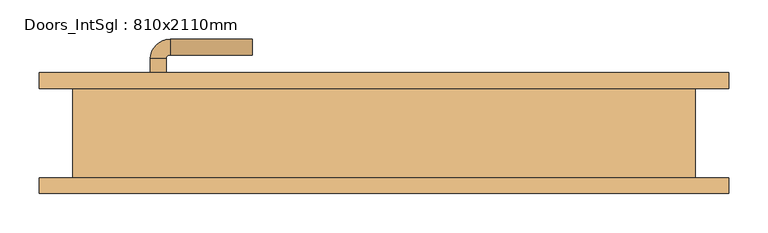
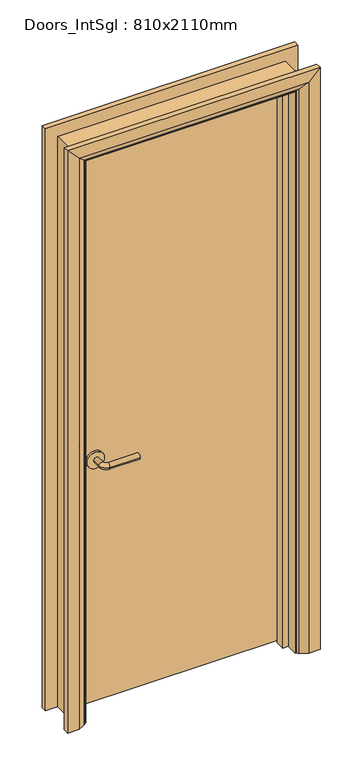
"""IFC4 building model written with IfcOpenShell, lengths in millimetres: door geometry, Doors_IntSgl : 810x2110mm."""

from ifc_helpers import new_model, si_unit, point, frame, frame_2d, origin, place, context, project, spatial, polyline, circle_curve, ellipse_curve, trimmed, segment, composite_curve, outline, extrude, faceted_brep, source, transform, mapped, element, save
from ifc_brep_helpers import plane_surface, cylinder_surface, revolved_surface, advanced_brep


def doors_intsgl_810x2110mm_5b69c0fd(model_context):
    return source(origin(), model_context, "Body", "SolidModel", [
        advanced_brep(
        [(-298.0, 11.15, 900.0), (-278.0, 11.15, 900.0), (-278.0, -18.85, 900.0), (-298.0, -18.85, 900.0), (-273.0, -23.85, 900.0), (-273.0, -43.85, 900.0), (-168.0, -43.85, 900.0), (-168.0, -23.85, 900.0)],
        [
            (0, 1, circle_curve(frame((-288.0, 11.15, 900.0), z_axis=(0.0, 1.0, 0.0), x_axis=(1.0, 0.0, 0.0)), 10.0)),
            (1, 0, circle_curve(frame((-288.0, 11.15, 900.0), z_axis=(0.0, 1.0, 0.0), x_axis=(1.0, 0.0, 0.0)), 10.0)),
            (1, 2),
            (2, 3, circle_curve(frame((-288.0, -18.85, 900.0), z_axis=(0.0, 1.0, 0.0), x_axis=(1.0, 0.0, 0.0)), 10.0)),
            (3, 0),
            (3, 2, circle_curve(frame((-288.0, -18.85, 900.0), z_axis=(0.0, 1.0, 0.0), x_axis=(1.0, 0.0, 0.0)), 10.0)),
            (4, 5, circle_curve(frame((-273.0, -33.85, 900.0), z_axis=(-1.0, 0.0, 0.0), x_axis=(0.0, 1.0, 0.0)), 10.0)),
            (5, 3, circle_curve(frame((-273.0, -18.85, 900.0), z_axis=(0.0, 0.0, -1.0), x_axis=(-1.0, 0.0, 0.0)), 25.0)),
            (2, 4, circle_curve(frame((-273.0, -18.85, 900.0), z_axis=(0.0, 0.0, 1.0), x_axis=(-1.0, 0.0, 0.0)), 5.0)),
            (5, 4, circle_curve(frame((-273.0, -33.85, 900.0), z_axis=(-1.0, 0.0, 0.0), x_axis=(0.0, 1.0, 0.0)), 10.0)),
            (6, 7, circle_curve(frame((-168.0, -33.85, 900.0), z_axis=(1.0, 0.0, 0.0), x_axis=(0.0, 1.0, 0.0)), 10.0)),
            (7, 6, circle_curve(frame((-168.0, -33.85, 900.0), z_axis=(1.0, 0.0, 0.0), x_axis=(0.0, 1.0, 0.0)), 10.0)),
            (4, 7),
            (6, 5),
        ],
        [
            plane_surface(frame((-288.0, 11.15, 900.0), z_axis=(0.0, 1.0, 0.0), x_axis=(0.0, 0.0, 1.0))),
            cylinder_surface(frame((-288.0, 11.15, 900.0), z_axis=(0.0, 1.0, 0.0), x_axis=(1.0, 0.0, 0.0)), 10.0),
            revolved_surface(trimmed(ellipse_curve(frame((-288.0, -18.85, 900.0), z_axis=(0.0, -1.0, 0.0), x_axis=(1.0, 0.0, 0.0)), 10.0, 10.0), [point((-298.0, -18.85, 900.0))], [point((-278.0, -18.85, 900.0))], True, "CARTESIAN"), (-273.0, -18.85, 900.0), (0.0, 0.0, -1.0)),
            revolved_surface(trimmed(ellipse_curve(frame((-288.0, -18.85, 900.0), z_axis=(0.0, -1.0, 0.0), x_axis=(1.0, 0.0, 0.0)), 10.0, 10.0), [point((-278.0, -18.85, 900.0))], [point((-298.0, -18.85, 900.0))], True, "CARTESIAN"), (-273.0, -18.85, 900.0), (0.0, 0.0, -1.0)),
            plane_surface(frame((-168.0, -33.85, 900.0), z_axis=(1.0, 0.0, 0.0), x_axis=(0.0, 0.0, 1.0))),
            cylinder_surface(frame((-273.0, -33.85, 900.0), z_axis=(-1.0, 0.0, 0.0), x_axis=(0.0, 1.0, 0.0)), 10.0),
        ],
        [
            (0, [[1, 2]]),
            (1, [[3, 4, 5, -2]]),
            (1, [[-5, 6, -3, -1]]),
            (2, [[7, 8, -4, 9]]),
            (3, [[10, -9, -6, -8]]),
            (4, [[11, 12]]),
            (5, [[13, -11, 14, -7]]),
            (5, [[-14, -12, -13, -10]]),
        ],
    ),
        extrude(outline(composite_curve([segment(trimmed(circle_curve(frame_2d((900.0, -290.5)), 30.0), [point((900.0, -320.5))], [point((900.0, -260.5))], False, "CARTESIAN"), True, "CONTINUOUS"), segment(trimmed(circle_curve(frame_2d((900.0, -290.5)), 30.0), [point((900.0, -260.5))], [point((900.0, -320.5))], False, "CARTESIAN"), True, "CONTINUOUS")], self_intersect=False)), frame((0.0, 11.15, 0.0), z_axis=(0.0, 1.0, 0.0), x_axis=(0.0, 0.0, 1.0)), (0.0, 0.0, 1.0), 8.0),
        advanced_brep(
        [(-298.0, 65.15, 900.0), (-278.0, 65.15, 900.0), (-298.0, 95.15, 900.0), (-278.0, 95.15, 900.0), (-273.0, 100.15, 900.0), (-273.0, 120.15, 900.0), (-168.0, 120.15, 900.0), (-168.0, 100.15, 900.0)],
        [
            (0, 1, circle_curve(frame((-288.0, 65.15, 900.0), z_axis=(0.0, -1.0, 0.0), x_axis=(1.0, 0.0, 0.0)), 10.0)),
            (1, 0, circle_curve(frame((-288.0, 65.15, 900.0), z_axis=(0.0, -1.0, 0.0), x_axis=(1.0, 0.0, 0.0)), 10.0)),
            (0, 2),
            (2, 3, circle_curve(frame((-288.0, 95.15, 900.0), z_axis=(0.0, -1.0, 0.0), x_axis=(1.0, 0.0, 0.0)), 10.0)),
            (3, 1),
            (3, 2, circle_curve(frame((-288.0, 95.15, 900.0), z_axis=(0.0, -1.0, 0.0), x_axis=(1.0, 0.0, 0.0)), 10.0)),
            (4, 3, circle_curve(frame((-273.0, 95.15, 900.0), z_axis=(0.0, 0.0, 1.0), x_axis=(-1.0, 0.0, 0.0)), 5.0)),
            (2, 5, circle_curve(frame((-273.0, 95.15, 900.0), z_axis=(0.0, 0.0, -1.0), x_axis=(-1.0, 0.0, 0.0)), 25.0)),
            (5, 4, circle_curve(frame((-273.0, 110.15, 900.0), z_axis=(-1.0, 0.0, 0.0), x_axis=(0.0, -1.0, 0.0)), 10.0)),
            (4, 5, circle_curve(frame((-273.0, 110.15, 900.0), z_axis=(-1.0, 0.0, 0.0), x_axis=(0.0, -1.0, 0.0)), 10.0)),
            (6, 7, circle_curve(frame((-168.0, 110.15, 900.0), z_axis=(1.0, 0.0, 0.0), x_axis=(0.0, -1.0, 0.0)), 10.0)),
            (7, 6, circle_curve(frame((-168.0, 110.15, 900.0), z_axis=(1.0, 0.0, 0.0), x_axis=(0.0, -1.0, 0.0)), 10.0)),
            (5, 6),
            (7, 4),
        ],
        [
            plane_surface(frame((-288.0, 65.15, 900.0), z_axis=(0.0, -1.0, 0.0), x_axis=(0.0, 0.0, 1.0))),
            cylinder_surface(frame((-288.0, 65.15, 900.0), z_axis=(0.0, -1.0, 0.0), x_axis=(1.0, 0.0, 0.0)), 10.0),
            revolved_surface(trimmed(ellipse_curve(frame((-288.0, 95.15, 900.0), z_axis=(0.0, -1.0, 0.0), x_axis=(1.0, 0.0, 0.0)), 10.0, 10.0), [point((-298.0, 95.15, 900.0))], [point((-278.0, 95.15, 900.0))], True, "CARTESIAN"), (-273.0, 95.15, 900.0), (0.0, 0.0, -1.0)),
            revolved_surface(trimmed(ellipse_curve(frame((-288.0, 95.15, 900.0), z_axis=(0.0, -1.0, 0.0), x_axis=(1.0, 0.0, 0.0)), 10.0, 10.0), [point((-278.0, 95.15, 900.0))], [point((-298.0, 95.15, 900.0))], True, "CARTESIAN"), (-273.0, 95.15, 900.0), (0.0, 0.0, -1.0)),
            plane_surface(frame((-168.0, 110.15, 900.0), z_axis=(1.0, 0.0, 0.0), x_axis=(0.0, 0.0, 1.0))),
            cylinder_surface(frame((-273.0, 110.15, 900.0), z_axis=(-1.0, 0.0, 0.0), x_axis=(0.0, -1.0, 0.0)), 10.0),
        ],
        [
            (0, [[1, 2]]),
            (1, [[-1, 3, 4, 5]]),
            (1, [[-2, -5, 6, -3]]),
            (2, [[7, -4, 8, 9]]),
            (3, [[-8, -6, -7, 10]]),
            (4, [[11, 12]]),
            (5, [[-9, 13, -12, 14]]),
            (5, [[-10, -14, -11, -13]]),
        ],
    ),
        extrude(outline(composite_curve([segment(trimmed(circle_curve(frame_2d((900.0, -290.5)), 30.0), [point((900.0, -320.5))], [point((900.0, -260.5))], False, "CARTESIAN"), True, "CONTINUOUS"), segment(trimmed(circle_curve(frame_2d((900.0, -290.5)), 30.0), [point((900.0, -260.5))], [point((900.0, -320.5))], False, "CARTESIAN"), True, "CONTINUOUS")], self_intersect=False)), frame((0.0, 57.15, 0.0), z_axis=(0.0, 1.0, 0.0), x_axis=(0.0, 0.0, 1.0)), (0.0, 0.0, 1.0), 8.0),
        extrude(outline(polyline([(363.0, 19.15), (-363.0, 19.15), (-363.0, 57.15), (363.0, 57.15), (363.0, 19.15)])), frame((0.0, 0.0, 8.0), z_axis=(0.0, 0.0, 1.0), x_axis=(1.0, 0.0, 0.0)), (0.0, 0.0, 1.0), 2060.0),
        advanced_brep(
        [(440.0, 77.15, 0.0), (440.0, 57.15, 0.0), (370.0, 57.15, 0.0), (374.0, 63.15, 0.0), (400.0, 77.15, 0.0), (440.0, 77.15, 2145.0), (440.0, 57.15, 2145.0), (-440.0, 57.15, 2145.0), (-440.0, 57.15, 0.0), (-370.0, 57.15, 0.0), (-370.0, 57.15, 2075.0), (370.0, 57.15, 2075.0), (374.0, 63.15, 2079.0), (400.0, 77.15, 2105.0), (-400.0, 77.15, 2105.0), (-400.0, 77.15, 0.0), (-440.0, 77.15, 0.0), (-440.0, 77.15, 2145.0), (-374.0, 63.15, 2079.0), (-374.0, 63.15, 0.0)],
        [
            (0, 1),
            (1, 2),
            (2, 3, circle_curve(frame((378.0, 56.15, 0.0), z_axis=(0.0, 0.0, -1.0), x_axis=(1.0, 0.0, 0.0)), 8.0622577)),
            (3, 4),
            (4, 0),
            (0, 5),
            (5, 6),
            (6, 1),
            (6, 7),
            (7, 8),
            (8, 9),
            (9, 10),
            (10, 11),
            (11, 2),
            (11, 12, ellipse_curve(frame((378.0, 56.15, 2083.0), z_axis=(0.7071067811865475, 0.0, -0.7071067811865475), x_axis=(-0.7071067811865474, 0.0, -0.7071067811865476)), 11.4017543, 8.0622577)),
            (12, 3),
            (12, 13),
            (13, 4),
            (13, 14),
            (14, 15),
            (15, 16),
            (16, 17),
            (17, 5),
            (17, 7),
            (10, 18, ellipse_curve(frame((-378.0, 56.15, 2083.0), z_axis=(0.7071067811865475, 0.0, 0.7071067811865475), x_axis=(0.7071067811865476, 0.0, -0.7071067811865474)), 11.4017543, 8.0622577)),
            (18, 12),
            (18, 14),
            (15, 19),
            (19, 9, circle_curve(frame((-378.0, 56.15, 0.0), z_axis=(0.0, 0.0, -1.0), x_axis=(-1.0, 0.0, 0.0)), 8.0622577)),
            (8, 16),
            (19, 18),
        ],
        [
            plane_surface(frame((370.0, 57.15, 0.0), z_axis=(0.0, 0.0, -1.0), x_axis=(0.0, -1.0, 0.0))),
            plane_surface(frame((440.0, 77.15, 0.0), z_axis=(1.0, 0.0, 0.0), x_axis=(0.0, 0.0, 1.0))),
            plane_surface(frame((440.0, 57.15, 0.0), z_axis=(0.0, -1.0, 0.0), x_axis=(0.0, 0.0, 1.0))),
            cylinder_surface(frame((378.0, 56.15, 0.0), z_axis=(0.0, 0.0, -1.0), x_axis=(1.0, 0.0, 0.0)), 8.0622577),
            plane_surface(frame((374.0, 63.15, 0.0), z_axis=(-0.4740998230350126, 0.880471099922178, 0.0), x_axis=(0.0, 0.0, 1.0))),
            plane_surface(frame((400.0, 77.15, 0.0), z_axis=(0.0, 1.0, 0.0), x_axis=(0.0, 0.0, 1.0))),
            plane_surface(frame((440.0, 77.15, 2145.0), z_axis=(0.0, 0.0, 1.0), x_axis=(-1.0, 0.0, 0.0))),
            cylinder_surface(frame((370.0, 56.15, 2083.0), z_axis=(1.0, 0.0, 0.0), x_axis=(0.0, 0.0, 1.0)), 8.0622577),
            plane_surface(frame((374.0, 63.15, 2079.0), z_axis=(0.0, 0.8804710999221764, -0.4740998230350154), x_axis=(-1.0, 0.0, 0.0))),
            plane_surface(frame((-370.0, 57.15, 0.0), z_axis=(0.0, 0.0, -1.0), x_axis=(0.0, -1.0, 0.0))),
            plane_surface(frame((-440.0, 77.15, 2145.0), z_axis=(-1.0, 0.0, 0.0), x_axis=(0.0, 0.0, -1.0))),
            cylinder_surface(frame((-378.0, 56.15, 2075.0), z_axis=(0.0, 0.0, 1.0), x_axis=(-1.0, 0.0, 0.0)), 8.0622577),
            plane_surface(frame((-374.0, 63.15, 2079.0), z_axis=(0.47409982303501824, 0.8804710999221749, 0.0), x_axis=(0.0, 0.0, -1.0))),
        ],
        [
            (0, [[1, 2, 3, 4, 5]]),
            (1, [[-1, 6, 7, 8]]),
            (2, [[-2, -8, 9, 10, 11, 12, 13, 14]]),
            (3, [[-3, -14, 15, 16]]),
            (4, [[-4, -16, 17, 18]]),
            (5, [[-5, -18, 19, 20, 21, 22, 23, -6]]),
            (6, [[-7, -23, 24, -9]]),
            (7, [[-15, -13, 25, 26]]),
            (8, [[-17, -26, 27, -19]]),
            (9, [[-21, 28, 29, -11, 30]]),
            (10, [[-24, -22, -30, -10]]),
            (11, [[-25, -12, -29, 31]]),
            (12, [[-27, -31, -28, -20]]),
        ],
    ),
        extrude(outline(polyline([(0.0, -365.0), (0.0, -346.0), (2051.0, -346.0), (2051.0, 346.0), (0.0, 346.0), (0.0, 365.0), (2070.0, 365.0), (2070.0, -365.0), (0.0, -365.0)])), frame((0.0, -14.85, 0.0), z_axis=(0.0, 1.0, 0.0), x_axis=(0.0, 0.0, 1.0)), (0.0, 0.0, 1.0), 32.0),
        advanced_brep(
        [(-440.0, -77.15, 0.0), (-440.0, -57.15, 0.0), (-370.0, -57.15, 0.0), (-374.0, -63.15, 0.0), (-400.0, -77.15, 0.0), (-440.0, -77.15, 2145.0), (-440.0, -57.15, 2145.0), (-370.0, -57.15, 2075.0), (-374.0, -63.15, 2079.0), (-400.0, -77.15, 2105.0), (440.0, -77.15, 2145.0), (440.0, -57.15, 2145.0), (370.0, -57.15, 2075.0), (374.0, -63.15, 2079.0), (400.0, -77.15, 2105.0), (440.0, -77.15, 0.0), (400.0, -77.15, 0.0), (374.0, -63.15, 0.0), (370.0, -57.15, 0.0), (440.0, -57.15, 0.0)],
        [
            (0, 1),
            (1, 2),
            (2, 3, circle_curve(frame((-378.0, -56.15, 0.0), z_axis=(0.0, 0.0, -1.0), x_axis=(-1.0, 0.0, 0.0)), 8.0622577)),
            (3, 4),
            (4, 0),
            (0, 5),
            (5, 6),
            (6, 1),
            (6, 7),
            (7, 2),
            (7, 8, ellipse_curve(frame((-378.0, -56.15, 2083.0), z_axis=(-0.7071067811865475, 0.0, -0.7071067811865475), x_axis=(0.7071067811865474, 0.0, -0.7071067811865476)), 11.4017543, 8.0622577)),
            (8, 3),
            (8, 9),
            (9, 4),
            (9, 5),
            (5, 10),
            (10, 11),
            (11, 6),
            (11, 12),
            (12, 7),
            (12, 13, ellipse_curve(frame((378.0, -56.15, 2083.0), z_axis=(-0.7071067811865475, 0.0, 0.7071067811865475), x_axis=(-0.7071067811865476, 0.0, -0.7071067811865474)), 11.4017543, 8.0622577)),
            (13, 8),
            (13, 14),
            (14, 9),
            (14, 10),
            (15, 16),
            (16, 17),
            (17, 18, circle_curve(frame((378.0, -56.15, 0.0), z_axis=(0.0, 0.0, -1.0), x_axis=(1.0, 0.0, 0.0)), 8.0622577)),
            (18, 19),
            (19, 15),
            (10, 15),
            (19, 11),
            (18, 12),
            (17, 13),
            (16, 14),
        ],
        [
            plane_surface(frame((-370.0, -129.9510989, 0.0), z_axis=(0.0, 0.0, -1.0), x_axis=(1.0, 0.0, 0.0))),
            plane_surface(frame((-440.0, -77.15, 0.0), z_axis=(-1.0, 0.0, 0.0), x_axis=(0.0, 0.0, 1.0))),
            plane_surface(frame((-440.0, -57.15, 0.0), z_axis=(0.0, 1.0, 0.0), x_axis=(0.0, 0.0, 1.0))),
            cylinder_surface(frame((-378.0, -56.15, 0.0), z_axis=(0.0, 0.0, -1.0), x_axis=(-1.0, 0.0, 0.0)), 8.0622577),
            plane_surface(frame((-374.0, -63.15, 0.0), z_axis=(0.4740998230350183, -0.8804710999221749, 0.0), x_axis=(0.0, 0.0, 1.0))),
            plane_surface(frame((-400.0, -77.15, 0.0), z_axis=(0.0, -1.0, 0.0), x_axis=(0.0, 0.0, 1.0))),
            plane_surface(frame((-440.0, -77.15, 2145.0), z_axis=(0.0, 0.0, 1.0), x_axis=(1.0, 0.0, 0.0))),
            plane_surface(frame((-440.0, -57.15, 2145.0), z_axis=(0.0, 1.0, 0.0), x_axis=(1.0, 0.0, 0.0))),
            cylinder_surface(frame((-370.0, -56.15, 2083.0), z_axis=(-1.0, 0.0, 0.0), x_axis=(0.0, 0.0, 1.0)), 8.0622577),
            plane_surface(frame((-374.0, -63.15, 2079.0), z_axis=(0.0, -0.8804710999221749, -0.4740998230350183), x_axis=(1.0, 0.0, 0.0))),
            plane_surface(frame((-400.0, -77.15, 2105.0), z_axis=(0.0, -1.0, 0.0), x_axis=(1.0, 0.0, 0.0))),
            plane_surface(frame((370.0, -129.9510989, 0.0), z_axis=(0.0, 0.0, -1.0), x_axis=(-1.0, 0.0, 0.0))),
            plane_surface(frame((440.0, -77.15, 2145.0), z_axis=(1.0, 0.0, 0.0), x_axis=(0.0, 0.0, -1.0))),
            plane_surface(frame((440.0, -57.15, 2145.0), z_axis=(0.0, 1.0, 0.0), x_axis=(0.0, 0.0, -1.0))),
            cylinder_surface(frame((378.0, -56.15, 2075.0), z_axis=(0.0, 0.0, 1.0), x_axis=(1.0, 0.0, 0.0)), 8.0622577),
            plane_surface(frame((374.0, -63.15, 2079.0), z_axis=(-0.4740998230350183, -0.8804710999221749, 0.0), x_axis=(0.0, 0.0, -1.0))),
            plane_surface(frame((400.0, -77.15, 2105.0), z_axis=(0.0, -1.0, 0.0), x_axis=(0.0, 0.0, -1.0))),
        ],
        [
            (0, [[1, 2, 3, 4, 5]]),
            (1, [[-1, 6, 7, 8]]),
            (2, [[-2, -8, 9, 10]]),
            (3, [[-3, -10, 11, 12]]),
            (4, [[-4, -12, 13, 14]]),
            (5, [[-5, -14, 15, -6]]),
            (6, [[-7, 16, 17, 18]]),
            (7, [[-9, -18, 19, 20]]),
            (8, [[-11, -20, 21, 22]]),
            (9, [[-13, -22, 23, 24]]),
            (10, [[-15, -24, 25, -16]]),
            (11, [[26, 27, 28, 29, 30]]),
            (12, [[-17, 31, -30, 32]]),
            (13, [[-19, -32, -29, 33]]),
            (14, [[-21, -33, -28, 34]]),
            (15, [[-23, -34, -27, 35]]),
            (16, [[-25, -35, -26, -31]]),
        ],
    ),
        faceted_brep([(-365.0, 57.15, 0.0), (-365.0, -57.15, 0.0), (-397.0, -57.15, 0.0), (-397.0, 57.15, 0.0), (-365.0, 57.15, 2070.0), (-365.0, -57.15, 2070.0), (-397.0, -57.15, 2102.0), (-397.0, 57.15, 2102.0), (365.0, 57.15, 2070.0), (365.0, -57.15, 2070.0), (397.0, -57.15, 2102.0), (397.0, 57.15, 2102.0), (365.0, 57.15, 0.0), (397.0, 57.15, 0.0), (397.0, -57.15, 0.0), (365.0, -57.15, 0.0)], [[[0, 1, 2, 3]], [[1, 0, 4, 5]], [[2, 1, 5, 6]], [[3, 2, 6, 7]], [[0, 3, 7, 4]], [[5, 4, 8, 9]], [[6, 5, 9, 10]], [[7, 6, 10, 11]], [[4, 7, 11, 8]], [[12, 13, 14, 15]], [[9, 8, 12, 15]], [[10, 9, 15, 14]], [[11, 10, 14, 13]], [[8, 11, 13, 12]]]),
    ])


if __name__ == "__main__":
    model = new_model("IFC4")
    model_context = context("Model", 3, world=origin())
    ifc_project = project(units=[si_unit("LENGTHUNIT", "METRE", prefix="MILLI")], contexts=[model_context])
    site = spatial("IfcSite", under=ifc_project)
    building = spatial("IfcBuilding", under=site)
    placement = place(None, origin())
    doors_intsgl_810x2110mm_shape = doors_intsgl_810x2110mm_5b69c0fd(model_context)
    element("IfcDoor", 1, ObjectType="Doors_IntSgl : 810x2110mm", at=placement, inside=building, context=model_context, shape_type="MappedRepresentation", body=[
        mapped(doors_intsgl_810x2110mm_shape, transform((0.0, 0.0, 0.0), x_axis=(1.0, 0.0, 0.0), y_axis=(0.0, 1.0, 0.0), z_axis=(0.0, 0.0, 1.0))),
    ])
    save(model, "model.ifc")

# Revit data of these elements
# Type "Doors_IntSgl : 810x2110mm"
#   Construction Type Id = "MDOOR"
#   Type Mark = "42"
#   Type Comments = "Internal Single"
#   Operation = "SingleSwingRight"
#   Manufacturer = "Revit"
#   Keynote = "L20"
#   Description = "Internal Single Door"
#   Analytic Construction = "Metal"
#   UnderCut = 0' - 0.31496"
#   Tolerance = 0' - 0.07874"
#   Thickness = 0' - 1.49606"
#   Thermal Resistance (R) = 0.270117 (m²·K)/W
#   Structural Tolerance = 0' - 0.31496"
#   StopDepth = 0' - 1.25984"
#   Stop Thickness = 0' - 0.74803"
#   Rough Width = 2' - 7.88976"
#   Rough Height = 6' - 11.07087"
#   Height to Top Lock Rail = 3' - 3.37008"
#   Heat Transfer Coefficient (U) = 3.7021 W/(m²·K)
#   Handle Z Distance = 2' - 11.43307"
#   Handle X Distance = 0' - 2.95276"
#   Frame Thickness = 0' - 1.25984"
#   Door Panel Width = 2' - 4.58268"
#   Door Panel Thickness = 0' - 1.49606"
#   Door Panel Offset = 0' - 0"
#   Height = 6' - 11.07087"
#   Width = 2' - 7.88976"
#   Door Panel Height = 6' - 9.10236"
#   Architrave Setback = 0' - 0.19685"
#   Define Thermal Properties by = 1
#   Vis - Ironmongery = yes
#   Material Ironmongery = Door - Handle
#   Material Frame = Door - Frame/Mullion (1)
#   Material Door = Door - Panel
#   Material Architrave = Door - Architrave
#   Visual Light Transmittance = 0
#   Solar Heat Gain Coefficient = 0
#   Function = (empty or 0)
#   Wall Closure = (empty or 0)
# Element 1 (IfcDoor, "Doors_IntSgl : 810x2110mm")
#   Materials on its faces: "Door - Architrave", "Door - Handle", "Door - Frame/Mullion (1)", "Door - Panel"
# Materials
#   "Door - Handle": colour RGB 17 17 17, transparency 0, Keynote = "P21", Cost = 0
#   "Door - Frame/Mullion (1)": class "Wood", colour RGB 212 179 113, transparency 0, Keynote = "L20", Cost = 0
#   "Door - Panel": class "Wood", colour RGB 210 159 95, transparency 0, Keynote = "L20", Cost = 0
#   "Door - Architrave": class "Wood", colour RGB 154 90 5, transparency 0, Keynote = "P20", Cost = 0
